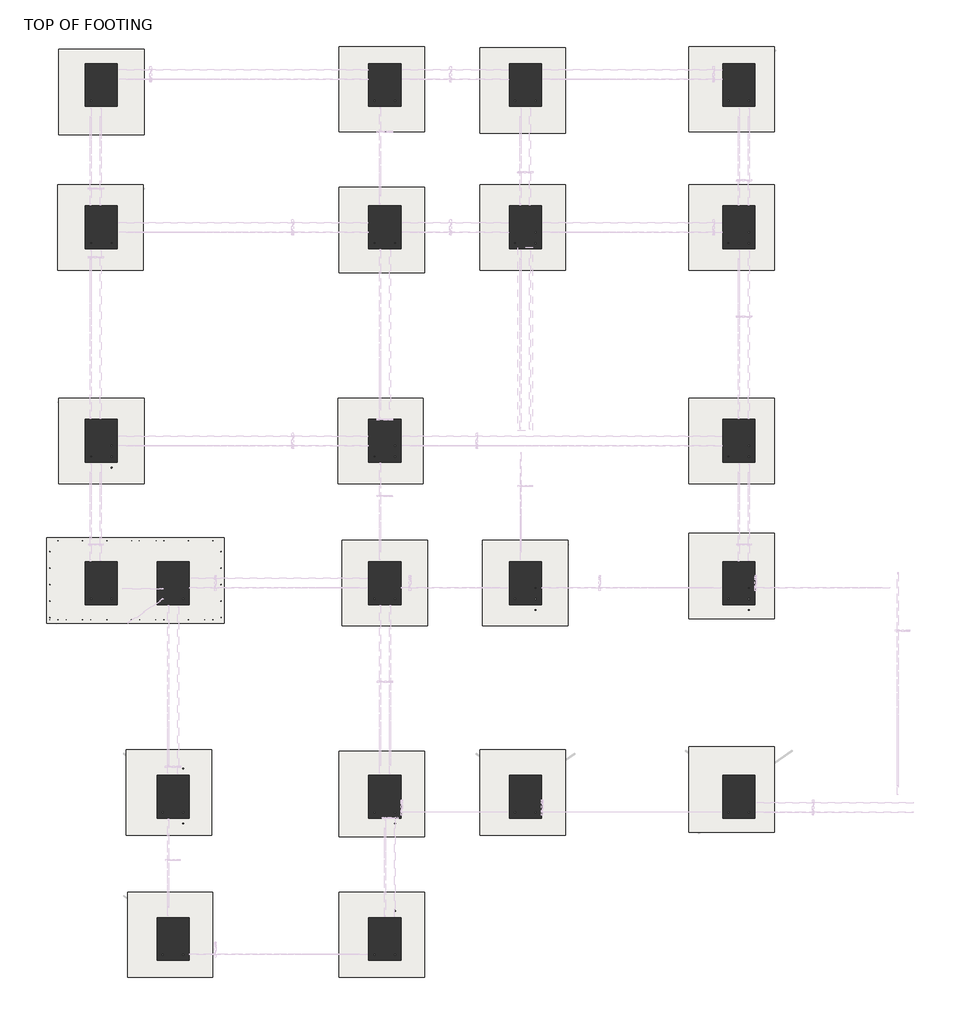
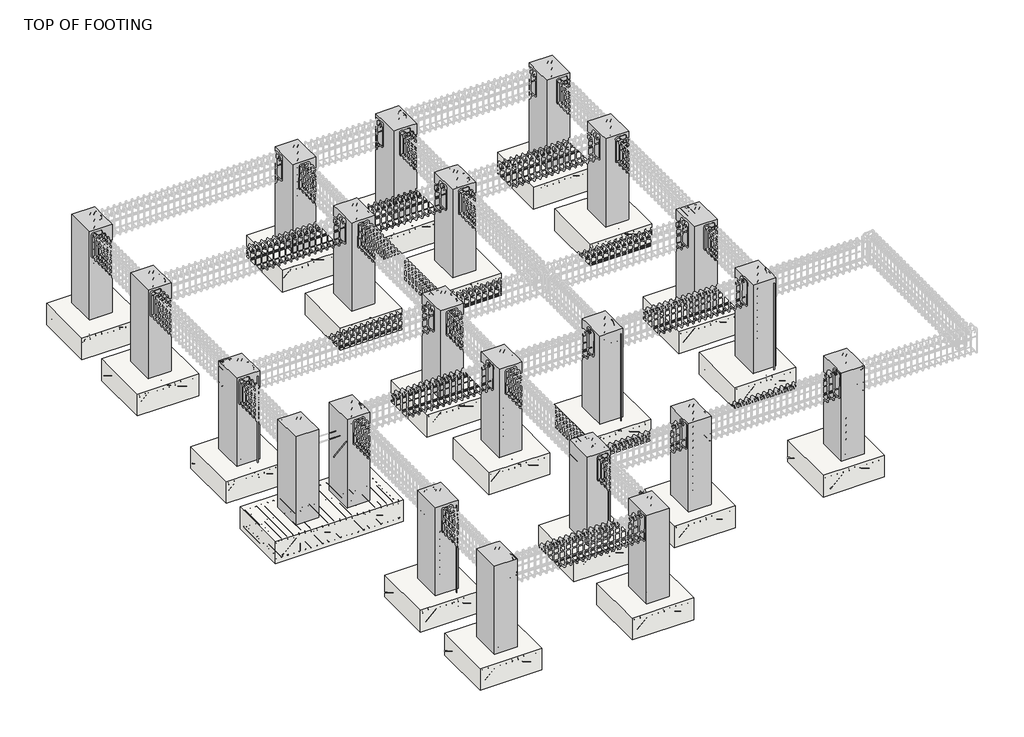
# One storey, part 1 of 17: 22 columns, 21 slabs.
"""IFC4 building model written with IfcOpenShell, lengths in millimetres."""

from ifc_helpers import new_model, si_unit, origin, place, context, project, spatial, faceted_brep, transform, mapped, element, save
from components import m_footing_rectangular_1200mmx1200mmx450mm_1789818b, m_footing_rectangular_1200mmx2500x450mm_3_75a58447

model = new_model("IFC4")

# Units and contexts
model_context = context("Model", 3, world=origin())
ifc_project = project(units=[si_unit("LENGTHUNIT", "METRE", prefix="MILLI")], contexts=[model_context])

# Site, building, storey
site = spatial("IfcSite", under=ifc_project)
building = spatial("IfcBuilding", under=site)
storey = spatial("IfcBuildingStorey", under=building, Name="TOP OF FOOTING", Elevation=-1828.8)

# Columns
placement = place(None, origin())
element("IfcColumn", 1, ObjectType="M_Concrete-Rectangular-Column : 450 x 600mm", at=placement, inside=storey, context=model_context, shape_type="Brep", body=[
    faceted_brep([(-4074.7920215, 9365.4757158, -1828.8), (-4074.7920215, 8765.4757158, -1828.8), (-4524.7920215, 8765.4757158, -1828.8), (-4524.7920215, 9365.4757158, -1828.8), (-4074.7920215, 9365.4757158, 0.0), (-4074.7920215, 9065.4757158, 0.0), (-4074.7920215, 8765.4757158, 0.0), (-4074.7920215, 8765.4757158, -300.0), (-4224.7920215, 8765.4757158, 0.0), (-4524.7920215, 8765.4757158, 0.0), (-4524.7920215, 9365.4757158, 0.0)], [[[0, 1, 2, 3]], [[1, 0, 4, 5, 6, 7]], [[2, 1, 7, 6, 8, 9]], [[3, 2, 9, 10]], [[0, 3, 10, 4]], [[10, 9, 8, 6, 5, 4]]]),
])
element("IfcColumn", 2, ObjectType="M_Concrete-Rectangular-Column : 450 x 600mm", at=placement, inside=storey, context=model_context, shape_type="Brep", body=[
    faceted_brep([(4887.1088658, 9365.4757158, -1828.8), (4887.1088658, 8765.4757158, -1828.8), (4437.1088658, 8765.4757158, -1828.8), (4437.1088658, 9365.4757158, -1828.8), (4887.1088658, 9365.4757158, 0.0), (4887.1088658, 8765.4757158, 0.0), (4587.1088658, 8765.4757158, 0.0), (4437.1088658, 8765.4757158, 0.0), (4437.1088658, 8765.4757158, -300.0), (4437.1088658, 9065.4757158, 0.0), (4437.1088658, 9365.4757158, 0.0)], [[[0, 1, 2, 3]], [[1, 0, 4, 5]], [[2, 1, 5, 6, 7, 8]], [[3, 2, 8, 7, 9, 10]], [[0, 3, 10, 4]], [[5, 4, 10, 9, 7, 6]]]),
])
element("IfcColumn", 3, ObjectType="M_Concrete-Rectangular-Column : 450 x 600mm", at=placement, inside=storey, context=model_context, shape_type="Brep", body=[
    faceted_brep([(1887.1088658, 9365.4757158, -1828.8), (1887.1088658, 8765.4757158, -1828.8), (1437.1088658, 8765.4757158, -1828.8), (1437.1088658, 9365.4757158, -1828.8), (1887.1088658, 9365.4757158, 0.0), (1887.1088658, 9065.4757158, 0.0), (1887.1088658, 8765.4757158, 0.0), (1887.1088658, 8765.4757158, -300.0), (1812.1088658, 8765.4757158, 0.0), (1512.1088658, 8765.4757158, 0.0), (1437.1088658, 8765.4757158, 0.0), (1437.1088658, 8765.4757158, -300.0), (1437.1088658, 9065.4757158, 0.0), (1437.1088658, 9365.4757158, 0.0)], [[[0, 1, 2, 3]], [[1, 0, 4, 5, 6, 7]], [[2, 1, 7, 6, 8, 9, 10, 11]], [[3, 2, 11, 10, 12, 13]], [[0, 3, 13, 4]], [[4, 13, 12, 10, 9, 8, 6, 5]]]),
])
element("IfcColumn", 4, ObjectType="M_Concrete-Rectangular-Column : 450 x 600mm", at=placement, inside=storey, context=model_context, shape_type="Brep", body=[
    faceted_brep([(-89.3669743, 9365.4757158, -1828.8), (-89.3669743, 8765.4757158, -1828.8), (-539.3669743, 8765.4757158, -1828.8), (-539.3669743, 9365.4757158, -1828.8), (-89.3669743, 9365.4757158, 0.0), (-89.3669743, 9065.4757158, 0.0), (-89.3669743, 8765.4757158, 0.0), (-89.3669743, 8765.4757158, -300.0), (-164.3669743, 8765.4757158, 0.0), (-464.3669743, 8765.4757158, 0.0), (-539.3669743, 8765.4757158, 0.0), (-539.3669743, 8765.4757158, -300.0), (-539.3669743, 9065.4757158, 0.0), (-539.3669743, 9365.4757158, 0.0)], [[[0, 1, 2, 3]], [[1, 0, 4, 5, 6, 7]], [[2, 1, 7, 6, 8, 9, 10, 11]], [[3, 2, 11, 10, 12, 13]], [[0, 3, 13, 4]], [[4, 13, 12, 10, 9, 8, 6, 5]]]),
])
element("IfcColumn", 5, ObjectType="M_Concrete-Rectangular-Column : 450 x 600mm", at=placement, inside=storey, context=model_context, shape_type="Brep", body=[
    faceted_brep([(-4074.7920215, 7365.4757158, -1828.8), (-4074.7920215, 6765.4757158, -1828.8), (-4524.7920215, 6765.4757158, -1828.8), (-4524.7920215, 7365.4757158, -1828.8), (-4074.7920215, 7365.4757158, -300.0), (-4074.7920215, 7365.4757158, 0.0), (-4074.7920215, 7215.4757158, 0.0), (-4074.7920215, 6915.4757158, 0.0), (-4074.7920215, 6765.4757158, 0.0), (-4074.7920215, 6765.4757158, -300.0), (-4224.7920215, 6765.4757158, 0.0), (-4524.7920215, 6765.4757158, 0.0), (-4524.7920215, 7365.4757158, 0.0), (-4224.7920215, 7365.4757158, 0.0)], [[[0, 1, 2, 3]], [[1, 0, 4, 5, 6, 7, 8, 9]], [[2, 1, 9, 8, 10, 11]], [[3, 2, 11, 12]], [[0, 3, 12, 13, 5, 4]], [[12, 11, 10, 8, 7, 6, 5, 13]]]),
])
element("IfcColumn", 6, ObjectType="M_Concrete-Rectangular-Column : 450 x 600mm", at=placement, inside=storey, context=model_context, shape_type="Brep", body=[
    faceted_brep([(-89.3669743, 7365.4757158, -1828.8), (-89.3669743, 6765.4757158, -1828.8), (-539.3669743, 6765.4757158, -1828.8), (-539.3669743, 7365.4757158, -1828.8), (-89.3669743, 7365.4757158, -300.0), (-89.3669743, 7365.4757158, 0.0), (-89.3669743, 7215.4757158, 0.0), (-89.3669743, 6915.4757158, 0.0), (-89.3669743, 6765.4757158, 0.0), (-89.3669743, 6765.4757158, -300.0), (-164.3669743, 6765.4757158, 0.0), (-464.3669743, 6765.4757158, 0.0), (-539.3669743, 6765.4757158, 0.0), (-539.3669743, 6765.4757158, -300.0), (-539.3669743, 6915.4757158, 0.0), (-539.3669743, 7215.4757158, 0.0), (-539.3669743, 7365.4757158, 0.0), (-539.3669743, 7365.4757158, -300.0), (-464.3669743, 7365.4757158, 0.0), (-164.3669743, 7365.4757158, 0.0)], [[[0, 1, 2, 3]], [[1, 0, 4, 5, 6, 7, 8, 9]], [[2, 1, 9, 8, 10, 11, 12, 13]], [[3, 2, 13, 12, 14, 15, 16, 17]], [[0, 3, 17, 16, 18, 19, 5, 4]], [[5, 19, 18, 16, 15, 14, 12, 11, 10, 8, 7, 6]]]),
])
element("IfcColumn", 7, ObjectType="M_Concrete-Rectangular-Column : 450 x 600mm", at=placement, inside=storey, context=model_context, shape_type="Brep", body=[
    faceted_brep([(1887.1088658, 7365.4757158, -1828.8), (1887.1088658, 6765.4757158, -1828.8), (1437.1088658, 6765.4757158, -1828.8), (1437.1088658, 7365.4757158, -1828.8), (1887.1088658, 7365.4757158, -300.0), (1887.1088658, 7365.4757158, 0.0), (1887.1088658, 7215.4757158, 0.0), (1887.1088658, 6915.4757158, 0.0), (1887.1088658, 6765.4757158, 0.0), (1887.1088658, 6765.4757158, -300.0), (1812.1088658, 6765.4757158, 0.0), (1512.1088658, 6765.4757158, 0.0), (1437.1088658, 6765.4757158, 0.0), (1437.1088658, 6765.4757158, -300.0), (1437.1088658, 6915.4757158, 0.0), (1437.1088658, 7215.4757158, 0.0), (1437.1088658, 7365.4757158, 0.0), (1437.1088658, 7365.4757158, -300.0), (1512.1088658, 7365.4757158, 0.0), (1812.1088658, 7365.4757158, 0.0)], [[[0, 1, 2, 3]], [[1, 0, 4, 5, 6, 7, 8, 9]], [[2, 1, 9, 8, 10, 11, 12, 13]], [[3, 2, 13, 12, 14, 15, 16, 17]], [[0, 3, 17, 16, 18, 19, 5, 4]], [[5, 19, 18, 16, 15, 14, 12, 11, 10, 8, 7, 6]]]),
])
element("IfcColumn", 8, ObjectType="M_Concrete-Rectangular-Column : 450 x 600mm", at=placement, inside=storey, context=model_context, shape_type="Brep", body=[
    faceted_brep([(4887.1088658, 7365.4757158, -1828.8), (4887.1088658, 6765.4757158, -1828.8), (4437.1088658, 6765.4757158, -1828.8), (4437.1088658, 7365.4757158, -1828.8), (4887.1088658, 7365.4757158, 0.0), (4887.1088658, 6765.4757158, 0.0), (4587.1088658, 6765.4757158, 0.0), (4437.1088658, 6765.4757158, 0.0), (4437.1088658, 6765.4757158, -300.0), (4437.1088658, 6915.4757158, 0.0), (4437.1088658, 7215.4757158, 0.0), (4437.1088658, 7365.4757158, 0.0), (4437.1088658, 7365.4757158, -300.0), (4587.1088658, 7365.4757158, 0.0)], [[[0, 1, 2, 3]], [[1, 0, 4, 5]], [[2, 1, 5, 6, 7, 8]], [[3, 2, 8, 7, 9, 10, 11, 12]], [[0, 3, 12, 11, 13, 4]], [[5, 4, 13, 11, 10, 9, 7, 6]]]),
])
element("IfcColumn", 9, ObjectType="M_Concrete-Rectangular-Column : 450 x 600mm", at=placement, inside=storey, context=model_context, shape_type="Brep", body=[
    faceted_brep([(-4074.7920215, 4365.4757158, -1828.8), (-4074.7920215, 3765.4757158, -1828.8), (-4524.7920215, 3765.4757158, -1828.8), (-4524.7920215, 4365.4757158, -1828.8), (-4074.7920215, 4365.4757158, -300.0), (-4074.7920215, 4365.4757158, 0.0), (-4074.7920215, 4215.4757158, 0.0), (-4074.7920215, 3915.4757158, 0.0), (-4074.7920215, 3765.4757158, 0.0), (-4074.7920215, 3765.4757158, -300.0), (-4224.7920215, 3765.4757158, 0.0), (-4524.7920215, 3765.4757158, 0.0), (-4524.7920215, 4365.4757158, 0.0), (-4224.7920215, 4365.4757158, 0.0)], [[[0, 1, 2, 3]], [[1, 0, 4, 5, 6, 7, 8, 9]], [[2, 1, 9, 8, 10, 11]], [[3, 2, 11, 12]], [[0, 3, 12, 13, 5, 4]], [[12, 11, 10, 8, 7, 6, 5, 13]]]),
])
element("IfcColumn", 10, ObjectType="M_Concrete-Rectangular-Column : 450 x 600mm", at=placement, inside=storey, context=model_context, shape_type="Brep", body=[
    faceted_brep([(4887.1088658, 4365.4757158, -1828.8), (4887.1088658, 3765.4757158, -1828.8), (4437.1088658, 3765.4757158, -1828.8), (4437.1088658, 4365.4757158, -1828.8), (4887.1088658, 4365.4757158, 0.0), (4887.1088658, 3765.4757158, 0.0), (4587.1088658, 3765.4757158, 0.0), (4437.1088658, 3765.4757158, 0.0), (4437.1088658, 3765.4757158, -300.0), (4437.1088658, 3915.4757158, 0.0), (4437.1088658, 4215.4757158, 0.0), (4437.1088658, 4365.4757158, 0.0), (4437.1088658, 4365.4757158, -300.0), (4587.1088658, 4365.4757158, 0.0)], [[[0, 1, 2, 3]], [[1, 0, 4, 5]], [[2, 1, 5, 6, 7, 8]], [[3, 2, 8, 7, 9, 10, 11, 12]], [[0, 3, 12, 11, 13, 4]], [[5, 4, 13, 11, 10, 9, 7, 6]]]),
])
element("IfcColumn", 11, ObjectType="M_Concrete-Rectangular-Column : 450 x 600mm", at=placement, inside=storey, context=model_context, shape_type="Brep", body=[
    faceted_brep([(-89.3669743, 4365.4757158, -1828.8), (-89.3669743, 3765.4757158, -1828.8), (-539.3669743, 3765.4757158, -1828.8), (-539.3669743, 4365.4757158, -1828.8), (-89.3669743, 4365.4757158, -300.0), (-89.3669743, 4365.4757158, 0.0), (-89.3669743, 4215.4757158, 0.0), (-89.3669743, 3915.4757158, 0.0), (-89.3669743, 3765.4757158, 0.0), (-89.3669743, 3765.4757158, -300.0), (-164.3669743, 3765.4757158, 0.0), (-464.3669743, 3765.4757158, 0.0), (-539.3669743, 3765.4757158, 0.0), (-539.3669743, 3765.4757158, -300.0), (-539.3669743, 3915.4757158, 0.0), (-539.3669743, 4215.4757158, 0.0), (-539.3669743, 4365.4757158, 0.0), (-539.3669743, 4365.4757158, -300.0), (-464.3669743, 4365.4757158, 0.0), (-164.3669743, 4365.4757158, 0.0)], [[[0, 1, 2, 3]], [[1, 0, 4, 5, 6, 7, 8, 9]], [[2, 1, 9, 8, 10, 11, 12, 13]], [[3, 2, 13, 12, 14, 15, 16, 17]], [[0, 3, 17, 16, 18, 19, 5, 4]], [[18, 16, 15, 14, 12, 11, 10, 8, 7, 6, 5, 19]]]),
])
element("IfcColumn", 12, ObjectType="M_Concrete-Rectangular-Column : 450 x 600mm", at=placement, inside=storey, context=model_context, shape_type="Brep", body=[
    faceted_brep([(-4074.7920215, 2365.4757158, -1828.8), (-4074.7920215, 1765.4757158, -1828.8), (-4524.7920215, 1765.4757158, -1828.8), (-4524.7920215, 2365.4757158, -1828.8), (-4074.7920215, 2365.4757158, -300.0), (-4074.7920215, 2365.4757158, 0.0), (-4074.7920215, 2215.4757158, 0.0), (-4074.7920215, 1765.4757158, 0.0), (-4524.7920215, 1765.4757158, 0.0), (-4524.7920215, 2365.4757158, 0.0), (-4224.7920215, 2365.4757158, 0.0)], [[[0, 1, 2, 3]], [[1, 0, 4, 5, 6, 7]], [[2, 1, 7, 8]], [[3, 2, 8, 9]], [[0, 3, 9, 10, 5, 4]], [[8, 7, 6, 5, 10, 9]]]),
])
element("IfcColumn", 13, ObjectType="M_Concrete-Rectangular-Column : 450 x 600mm", at=placement, inside=storey, context=model_context, shape_type="Brep", body=[
    faceted_brep([(-3067.007124, 2365.4757158, -1828.8), (-3067.007124, 1765.4757158, -1828.8), (-3517.007124, 1765.4757158, -1828.8), (-3517.007124, 2365.4757158, -1828.8), (-3067.007124, 2365.4757158, -300.0), (-3067.007124, 2365.4757158, 0.0), (-3067.007124, 2215.4757158, 0.0), (-3067.007124, 1915.4757158, 0.0), (-3067.007124, 1765.4757158, 0.0), (-3067.007124, 1765.4757158, -300.0), (-3142.007124, 1765.4757158, 0.0), (-3517.007124, 1765.4757158, 0.0), (-3517.007124, 2215.4757158, 0.0), (-3517.007124, 2365.4757158, 0.0), (-3517.007124, 2365.4757158, -300.0)], [[[0, 1, 2, 3]], [[1, 0, 4, 5, 6, 7, 8, 9]], [[2, 1, 9, 8, 10, 11]], [[3, 2, 11, 12, 13, 14]], [[0, 3, 14, 13, 5, 4]], [[5, 13, 12, 11, 10, 8, 7, 6]]]),
])
element("IfcColumn", 14, ObjectType="M_Concrete-Rectangular-Column : 450 x 600mm", at=placement, inside=storey, context=model_context, shape_type="Brep", body=[
    faceted_brep([(-89.3669743, 2365.4757158, -1828.8), (-89.3669743, 1765.4757158, -1828.8), (-539.3669743, 1765.4757158, -1828.8), (-539.3669743, 2365.4757158, -1828.8), (-89.3669743, 2365.4757158, -300.0), (-89.3669743, 2365.4757158, 0.0), (-89.3669743, 2215.4757158, 0.0), (-89.3669743, 1915.4757158, 0.0), (-89.3669743, 1765.4757158, 0.0), (-89.3669743, 1765.4757158, -300.0), (-164.3669743, 1765.4757158, 0.0), (-464.3669743, 1765.4757158, 0.0), (-539.3669743, 1765.4757158, 0.0), (-539.3669743, 1765.4757158, -300.0), (-539.3669743, 1915.4757158, 0.0), (-539.3669743, 2215.4757158, 0.0), (-539.3669743, 2365.4757158, 0.0), (-539.3669743, 2365.4757158, -300.0), (-464.3669743, 2365.4757158, 0.0), (-164.3669743, 2365.4757158, 0.0)], [[[0, 1, 2, 3]], [[1, 0, 4, 5, 6, 7, 8, 9]], [[2, 1, 9, 8, 10, 11, 12, 13]], [[3, 2, 13, 12, 14, 15, 16, 17]], [[0, 3, 17, 16, 18, 19, 5, 4]], [[18, 16, 15, 14, 12, 11, 10, 8, 7, 6, 5, 19]]]),
])
element("IfcColumn", 15, ObjectType="M_Concrete-Rectangular-Column : 450 x 600mm", at=placement, inside=storey, context=model_context, shape_type="Brep", body=[
    faceted_brep([(4887.1088658, 2365.4757158, -1828.8), (4887.1088658, 1765.4757158, -1828.8), (4437.1088658, 1765.4757158, -1828.8), (4437.1088658, 2365.4757158, -1828.8), (4887.1088658, 2365.4757158, 0.0), (4887.1088658, 1915.4757158, 0.0), (4887.1088658, 1765.4757158, 0.0), (4887.1088658, 1765.4757158, -300.0), (4437.1088658, 1765.4757158, 0.0), (4437.1088658, 1765.4757158, -300.0), (4437.1088658, 1915.4757158, 0.0), (4437.1088658, 2215.4757158, 0.0), (4437.1088658, 2365.4757158, 0.0), (4437.1088658, 2365.4757158, -300.0), (4587.1088658, 2365.4757158, 0.0)], [[[0, 1, 2, 3]], [[1, 0, 4, 5, 6, 7]], [[2, 1, 7, 6, 8, 9]], [[3, 2, 9, 8, 10, 11, 12, 13]], [[0, 3, 13, 12, 14, 4]], [[8, 6, 5, 4, 14, 12, 11, 10]]]),
])
element("IfcColumn", 16, ObjectType="M_Concrete-Rectangular-Column : 450 x 600mm", at=placement, inside=storey, context=model_context, shape_type="Brep", body=[
    faceted_brep([(1887.1088658, 2365.4757158, -1828.8), (1887.1088658, 1765.4757158, -1828.8), (1437.1088658, 1765.4757158, -1828.8), (1437.1088658, 2365.4757158, -1828.8), (1887.1088658, 2365.4757158, -300.0), (1887.1088658, 2365.4757158, 0.0), (1887.1088658, 2215.4757158, 0.0), (1887.1088658, 1915.4757158, 0.0), (1887.1088658, 1765.4757158, 0.0), (1887.1088658, 1765.4757158, -300.0), (1437.1088658, 1765.4757158, 0.0), (1437.1088658, 1765.4757158, -300.0), (1437.1088658, 1915.4757158, 0.0), (1437.1088658, 2215.4757158, 0.0), (1437.1088658, 2365.4757158, 0.0), (1437.1088658, 2365.4757158, -300.0), (1512.1088658, 2365.4757158, 0.0), (1812.1088658, 2365.4757158, 0.0)], [[[0, 1, 2, 3]], [[1, 0, 4, 5, 6, 7, 8, 9]], [[2, 1, 9, 8, 10, 11]], [[3, 2, 11, 10, 12, 13, 14, 15]], [[0, 3, 15, 14, 16, 17, 5, 4]], [[10, 8, 7, 6, 5, 17, 16, 14, 13, 12]]]),
])
element("IfcColumn", 17, ObjectType="M_Concrete-Rectangular-Column : 450 x 600mm", at=placement, inside=storey, context=model_context, shape_type="Brep", body=[
    faceted_brep([(-3067.007124, -634.5242842, -1828.8), (-3067.007124, -1234.5242842, -1828.8), (-3517.007124, -1234.5242842, -1828.8), (-3517.007124, -634.5242842, -1828.8), (-3067.007124, -634.5242842, -300.0), (-3067.007124, -634.5242842, 0.0), (-3067.007124, -1234.5242842, 0.0), (-3067.007124, -1234.5242842, -300.0), (-3142.007124, -1234.5242842, 0.0), (-3517.007124, -1234.5242842, 0.0), (-3517.007124, -634.5242842, 0.0), (-3142.007124, -634.5242842, 0.0)], [[[0, 1, 2, 3]], [[1, 0, 4, 5, 6, 7]], [[2, 1, 7, 6, 8, 9]], [[3, 2, 9, 10]], [[0, 3, 10, 11, 5, 4]], [[6, 5, 11, 10, 9, 8]]]),
])
element("IfcColumn", 18, ObjectType="M_Concrete-Rectangular-Column : 450 x 600mm", at=placement, inside=storey, context=model_context, shape_type="Brep", body=[
    faceted_brep([(4887.1088658, -634.5242842, -1828.8), (4887.1088658, -1234.5242842, -1828.8), (4437.1088658, -1234.5242842, -1828.8), (4437.1088658, -634.5242842, -1828.8), (4887.1088658, -634.5242842, -300.0), (4887.1088658, -634.5242842, 0.0), (4887.1088658, -934.5242842, 0.0), (4887.1088658, -1234.5242842, 0.0), (4437.1088658, -1234.5242842, 0.0), (4437.1088658, -934.5242842, 0.0), (4437.1088658, -634.5242842, 0.0), (4437.1088658, -634.5242842, -300.0)], [[[0, 1, 2, 3]], [[1, 0, 4, 5, 6, 7]], [[2, 1, 7, 8]], [[3, 2, 8, 9, 10, 11]], [[0, 3, 11, 10, 5, 4]], [[8, 7, 6, 5, 10, 9]]]),
])
element("IfcColumn", 19, ObjectType="M_Concrete-Rectangular-Column : 450 x 600mm", at=placement, inside=storey, context=model_context, shape_type="Brep", body=[
    faceted_brep([(1887.1088658, -634.5242842, -1828.8), (1887.1088658, -1234.5242842, -1828.8), (1437.1088658, -1234.5242842, -1828.8), (1437.1088658, -634.5242842, -1828.8), (1887.1088658, -634.5242842, -300.0), (1887.1088658, -634.5242842, 0.0), (1887.1088658, -934.5242842, 0.0), (1887.1088658, -1234.5242842, 0.0), (1437.1088658, -1234.5242842, 0.0), (1437.1088658, -934.5242842, 0.0), (1437.1088658, -634.5242842, 0.0), (1437.1088658, -634.5242842, -300.0)], [[[0, 1, 2, 3]], [[1, 0, 4, 5, 6, 7]], [[2, 1, 7, 8]], [[3, 2, 8, 9, 10, 11]], [[0, 3, 11, 10, 5, 4]], [[8, 7, 6, 5, 10, 9]]]),
])
element("IfcColumn", 20, ObjectType="M_Concrete-Rectangular-Column : 450 x 600mm", at=placement, inside=storey, context=model_context, shape_type="Brep", body=[
    faceted_brep([(-89.3669743, -634.5242842, -1828.8), (-89.3669743, -1234.5242842, -1828.8), (-539.3669743, -1234.5242842, -1828.8), (-539.3669743, -634.5242842, -1828.8), (-89.3669743, -634.5242842, -300.0), (-89.3669743, -634.5242842, 0.0), (-89.3669743, -934.5242842, 0.0), (-89.3669743, -1234.5242842, 0.0), (-389.3669743, -1234.5242842, 0.0), (-539.3669743, -1234.5242842, 0.0), (-539.3669743, -1234.5242842, -300.0), (-539.3669743, -634.5242842, 0.0), (-539.3669743, -634.5242842, -300.0), (-464.3669743, -634.5242842, 0.0), (-164.3669743, -634.5242842, 0.0)], [[[0, 1, 2, 3]], [[1, 0, 4, 5, 6, 7]], [[2, 1, 7, 8, 9, 10]], [[3, 2, 10, 9, 11, 12]], [[0, 3, 12, 11, 13, 14, 5, 4]], [[11, 9, 8, 7, 6, 5, 14, 13]]]),
])
element("IfcColumn", 21, ObjectType="M_Concrete-Rectangular-Column : 450 x 600mm", at=placement, inside=storey, context=model_context, shape_type="Brep", body=[
    faceted_brep([(-3067.007124, -2634.5242842, -1828.8), (-3067.007124, -3234.5242842, -1828.8), (-3517.007124, -3234.5242842, -1828.8), (-3517.007124, -2634.5242842, -1828.8), (-3067.007124, -2634.5242842, -300.0), (-3067.007124, -2634.5242842, 0.0), (-3067.007124, -2934.5242842, 0.0), (-3067.007124, -3234.5242842, 0.0), (-3517.007124, -3234.5242842, 0.0), (-3517.007124, -2634.5242842, 0.0), (-3142.007124, -2634.5242842, 0.0)], [[[0, 1, 2, 3]], [[1, 0, 4, 5, 6, 7]], [[2, 1, 7, 8]], [[3, 2, 8, 9]], [[0, 3, 9, 10, 5, 4]], [[8, 7, 6, 5, 10, 9]]]),
])
element("IfcColumn", 22, ObjectType="M_Concrete-Rectangular-Column : 450 x 600mm", at=placement, inside=storey, context=model_context, shape_type="Brep", body=[
    faceted_brep([(-89.3669743, -2634.5242842, -1828.8), (-89.3669743, -3234.5242842, -1828.8), (-539.3669743, -3234.5242842, -1828.8), (-539.3669743, -2634.5242842, -1828.8), (-89.3669743, -2634.5242842, 0.0), (-89.3669743, -3234.5242842, 0.0), (-539.3669743, -3234.5242842, 0.0), (-539.3669743, -2934.5242842, 0.0), (-539.3669743, -2634.5242842, 0.0), (-539.3669743, -2634.5242842, -300.0), (-389.3669743, -2634.5242842, 0.0)], [[[0, 1, 2, 3]], [[1, 0, 4, 5]], [[2, 1, 5, 6]], [[3, 2, 6, 7, 8, 9]], [[0, 3, 9, 8, 10, 4]], [[5, 4, 10, 8, 7, 6]]]),
])

# Slabs
m_footing_rectangular_1200mmx1200mmx450mm_shape = m_footing_rectangular_1200mmx1200mmx450mm_1789818b(model_context)
element("IfcSlab", 23, ObjectType="M_Footing-Rectangular : 1200MMX1200MMX450MM", at=placement, inside=storey, context=model_context, shape_type="MappedRepresentation", body=[
    mapped(m_footing_rectangular_1200mmx1200mmx450mm_shape, transform((-4299.7920215, 8965.4757158, -1828.8), x_axis=(1.0, 0.0, 0.0), y_axis=(0.0, 1.0, 0.0), z_axis=(0.0, 0.0, 1.0))),
])
element("IfcSlab", 24, ObjectType="M_Footing-Rectangular : 1200MMX1200MMX450MM", at=placement, inside=storey, context=model_context, shape_type="MappedRepresentation", body=[
    mapped(m_footing_rectangular_1200mmx1200mmx450mm_shape, transform((-354.3669743, 9005.4757158, -1828.8), x_axis=(1.0, 0.0, 0.0), y_axis=(0.0, 1.0, 0.0), z_axis=(0.0, 0.0, 1.0))),
])
element("IfcSlab", 25, ObjectType="M_Footing-Rectangular : 1200MMX1200MMX450MM", at=placement, inside=storey, context=model_context, shape_type="MappedRepresentation", body=[
    mapped(m_footing_rectangular_1200mmx1200mmx450mm_shape, transform((1622.1088658, 8985.4757158, -1828.8), x_axis=(1.0, 0.0, 0.0), y_axis=(0.0, 1.0, 0.0), z_axis=(0.0, 0.0, 1.0))),
])
element("IfcSlab", 26, ObjectType="M_Footing-Rectangular : 1200MMX1200MMX450MM", at=placement, inside=storey, context=model_context, shape_type="MappedRepresentation", body=[
    mapped(m_footing_rectangular_1200mmx1200mmx450mm_shape, transform((4562.1088658, 9005.4757158, -1828.8), x_axis=(1.0, 0.0, 0.0), y_axis=(0.0, 1.0, 0.0), z_axis=(0.0, 0.0, 1.0))),
])
element("IfcSlab", 27, ObjectType="M_Footing-Rectangular : 1200MMX1200MMX450MM", at=placement, inside=storey, context=model_context, shape_type="MappedRepresentation", body=[
    mapped(m_footing_rectangular_1200mmx1200mmx450mm_shape, transform((-4312.007124, 7065.4757158, -1828.8), x_axis=(1.0, 0.0, 0.0), y_axis=(0.0, 1.0, 0.0), z_axis=(0.0, 0.0, 1.0))),
])
element("IfcSlab", 28, ObjectType="M_Footing-Rectangular : 1200MMX1200MMX450MM", at=placement, inside=storey, context=model_context, shape_type="MappedRepresentation", body=[
    mapped(m_footing_rectangular_1200mmx1200mmx450mm_shape, transform((-4299.7920215, 4065.4757158, -1828.8), x_axis=(1.0, 0.0, 0.0), y_axis=(0.0, 1.0, 0.0), z_axis=(0.0, 0.0, 1.0))),
])
element("IfcSlab", 29, ObjectType="M_Footing-Rectangular : 1200MMX1200MMX450MM", at=placement, inside=storey, context=model_context, shape_type="MappedRepresentation", body=[
    mapped(m_footing_rectangular_1200mmx1200mmx450mm_shape, transform((-314.3669743, 2065.4757158, -1828.8), x_axis=(1.0, 0.0, 0.0), y_axis=(0.0, 1.0, 0.0), z_axis=(0.0, 0.0, 1.0))),
])
element("IfcSlab", 30, ObjectType="M_Footing-Rectangular : 1200MMX1200MMX450MM", at=placement, inside=storey, context=model_context, shape_type="MappedRepresentation", body=[
    mapped(m_footing_rectangular_1200mmx1200mmx450mm_shape, transform((1662.1088658, 2065.4757158, -1828.8), x_axis=(1.0, 0.0, 0.0), y_axis=(0.0, 1.0, 0.0), z_axis=(0.0, 0.0, 1.0))),
])
element("IfcSlab", 31, ObjectType="M_Footing-Rectangular : 1200MMX1200MMX450MM", at=placement, inside=storey, context=model_context, shape_type="MappedRepresentation", body=[
    mapped(m_footing_rectangular_1200mmx1200mmx450mm_shape, transform((4562.1088658, 2165.4757158, -1828.8), x_axis=(1.0, 0.0, 0.0), y_axis=(0.0, 1.0, 0.0), z_axis=(0.0, 0.0, 1.0))),
])
element("IfcSlab", 32, ObjectType="M_Footing-Rectangular : 1200MMX1200MMX450MM", at=placement, inside=storey, context=model_context, shape_type="MappedRepresentation", body=[
    mapped(m_footing_rectangular_1200mmx1200mmx450mm_shape, transform((4562.1088658, -834.5242842, -1828.8), x_axis=(1.0, 0.0, 0.0), y_axis=(0.0, 1.0, 0.0), z_axis=(0.0, 0.0, 1.0))),
])
element("IfcSlab", 33, ObjectType="M_Footing-Rectangular : 1200MMX1200MMX450MM", at=placement, inside=storey, context=model_context, shape_type="MappedRepresentation", body=[
    mapped(m_footing_rectangular_1200mmx1200mmx450mm_shape, transform((1622.1088658, -874.5242842, -1828.8), x_axis=(1.0, 0.0, 0.0), y_axis=(0.0, 1.0, 0.0), z_axis=(0.0, 0.0, 1.0))),
])
element("IfcSlab", 34, ObjectType="M_Footing-Rectangular : 1200MMX1200MMX450MM", at=placement, inside=storey, context=model_context, shape_type="MappedRepresentation", body=[
    mapped(m_footing_rectangular_1200mmx1200mmx450mm_shape, transform((-354.3669743, -894.5242842, -1828.8), x_axis=(1.0, 0.0, 0.0), y_axis=(0.0, 1.0, 0.0), z_axis=(0.0, 0.0, 1.0))),
])
element("IfcSlab", 35, ObjectType="M_Footing-Rectangular : 1200MMX1200MMX450MM", at=placement, inside=storey, context=model_context, shape_type="MappedRepresentation", body=[
    mapped(m_footing_rectangular_1200mmx1200mmx450mm_shape, transform((-3352.007124, -874.5242842, -1828.8), x_axis=(1.0, 0.0, 0.0), y_axis=(0.0, 1.0, 0.0), z_axis=(0.0, 0.0, 1.0))),
])
element("IfcSlab", 36, ObjectType="M_Footing-Rectangular : 1200MMX1200MMX450MM", at=placement, inside=storey, context=model_context, shape_type="MappedRepresentation", body=[
    mapped(m_footing_rectangular_1200mmx1200mmx450mm_shape, transform((-3332.007124, -2874.5242842, -1828.8), x_axis=(1.0, 0.0, 0.0), y_axis=(0.0, 1.0, 0.0), z_axis=(0.0, 0.0, 1.0))),
])
element("IfcSlab", 37, ObjectType="M_Footing-Rectangular : 1200MMX1200MMX450MM", at=placement, inside=storey, context=model_context, shape_type="MappedRepresentation", body=[
    mapped(m_footing_rectangular_1200mmx1200mmx450mm_shape, transform((-354.3669743, -2874.5242842, -1828.8), x_axis=(1.0, 0.0, 0.0), y_axis=(0.0, 1.0, 0.0), z_axis=(0.0, 0.0, 1.0))),
])
element("IfcSlab", 38, ObjectType="M_Footing-Rectangular : 1200MMX1200MMX450MM", at=placement, inside=storey, context=model_context, shape_type="MappedRepresentation", body=[
    mapped(m_footing_rectangular_1200mmx1200mmx450mm_shape, transform((-374.3669743, 4065.4757158, -1828.8), x_axis=(1.0, 0.0, 0.0), y_axis=(0.0, 1.0, 0.0), z_axis=(0.0, 0.0, 1.0))),
])
element("IfcSlab", 39, ObjectType="M_Footing-Rectangular : 1200MMX1200MMX450MM", at=placement, inside=storey, context=model_context, shape_type="MappedRepresentation", body=[
    mapped(m_footing_rectangular_1200mmx1200mmx450mm_shape, transform((4562.1088658, 4065.4757158, -1828.8), x_axis=(1.0, 0.0, 0.0), y_axis=(0.0, 1.0, 0.0), z_axis=(0.0, 0.0, 1.0))),
])
element("IfcSlab", 40, ObjectType="M_Footing-Rectangular : 1200MMX1200MMX450MM", at=placement, inside=storey, context=model_context, shape_type="MappedRepresentation", body=[
    mapped(m_footing_rectangular_1200mmx1200mmx450mm_shape, transform((4562.1088658, 7065.4757158, -1828.8), x_axis=(1.0, 0.0, 0.0), y_axis=(0.0, 1.0, 0.0), z_axis=(0.0, 0.0, 1.0))),
])
element("IfcSlab", 41, ObjectType="M_Footing-Rectangular : 1200MMX1200MMX450MM", at=placement, inside=storey, context=model_context, shape_type="MappedRepresentation", body=[
    mapped(m_footing_rectangular_1200mmx1200mmx450mm_shape, transform((1622.1088658, 7065.4757158, -1828.8), x_axis=(1.0, 0.0, 0.0), y_axis=(0.0, 1.0, 0.0), z_axis=(0.0, 0.0, 1.0))),
])
element("IfcSlab", 42, ObjectType="M_Footing-Rectangular : 1200MMX1200MMX450MM", at=placement, inside=storey, context=model_context, shape_type="MappedRepresentation", body=[
    mapped(m_footing_rectangular_1200mmx1200mmx450mm_shape, transform((-354.3669743, 7025.4757158, -1828.8), x_axis=(1.0, 0.0, 0.0), y_axis=(0.0, 1.0, 0.0), z_axis=(0.0, 0.0, 1.0))),
])
m_footing_rectangular_1200mmx2500x450mm_3_shape = m_footing_rectangular_1200mmx2500x450mm_3_75a58447(model_context)
element("IfcSlab", 43, ObjectType="M_Footing-Rectangular : 1200MMX2500X450MM 3", at=placement, inside=storey, context=model_context, shape_type="MappedRepresentation", body=[
    mapped(m_footing_rectangular_1200mmx2500x450mm_3_shape, transform((-3819.7920215, 2105.4757158, -1828.8), x_axis=(0.0, 1.0, 0.0), y_axis=(-1.0, 0.0, 0.0), z_axis=(0.0, 0.0, 1.0))),
])

save(model, "model.ifc")

# Revit data of these elements
# Grids (mm)
#   "1": line (-4299.792, -7551.18) -> (-4299.792, 10278.991)
#   "3": line (-1299.792, -7551.18) -> (-1299.792, 10278.991)
#   "4": line (-314.367, -7551.18) -> (-314.367, 10429.888)
#   "5": line (1662.109, -7551.18) -> (1662.109, 11644.031)
#   "6": line (4662.109, -7551.18) -> (4662.109, 11644.031)
#   "2": line (-3292.007, -7551.18) -> (-3292.007, 11644.031)
#   "A": line (9910.38, 9065.476) -> (-6361.637, 9065.476)
#   "B": line (9910.38, 7065.476) -> (-6361.637, 7065.476)
#   "C": line (9910.38, 4065.476) -> (-6361.637, 4065.476)
#   "D": line (9910.38, 2065.476) -> (-6361.637, 2065.476)
#   "E": line (9910.38, -934.524) -> (-6361.637, -934.524)
#   "F": line (9910.38, -2934.524) -> (-6361.637, -2934.524)
# Type "M_Concrete-Rectangular-Column : 450 x 600mm"
#   b = 450 mm
#   h = 600 mm
#   Structural Material [instance default] = Concrete, Cast-in-Place gray
# Type "M_Footing-Rectangular : 1200MMX1200MMX450MM"
#   Width = 1200 mm
#   Length = 1200 mm
#   Foundation Thickness = 450 mm
#   Structural Material [instance default] = Concrete, Cast-in-Place gray
#   Assembly Code = ""
# Type "M_Footing-Rectangular : 1200MMX2500X450MM 3"
#   Width = 1200 mm
#   Length = 2500 mm
#   Foundation Thickness = 450 mm
#   Structural Material [instance default] = Concrete, Cast-in-Place gray
#   Assembly Code = ""
# Elements 1, 2, 3, 4, 5, 6, 7, 8, 9, 10, 11, 12, 13, 14, 15, 16, 17, 18, 19, 20, 21, 22 (IfcColumn, "M_Concrete-Rectangular-Column : 450 x 600mm")
#   Structural Material = Concrete, Cast-in-Place gray
#   Phase Created = New Construction
#   Materials on its faces: "Concrete, Cast-in-Place gray"
# Elements 23, 24, 25, 26, 27, 28, 29, 30, 31, 32, 33, 34, 35, 36, 37, 38, 39, 40, 41, 42 (IfcSlab, "M_Footing-Rectangular : 1200MMX1200MMX450MM")
#   Structural Material = Concrete, Cast-in-Place gray
#   Phase Created = New Construction
#   Materials on its faces: "Concrete, Cast-in-Place gray"
# Element 43 (IfcSlab, "M_Footing-Rectangular : 1200MMX2500X450MM 3")
#   Structural Material = Concrete, Cast-in-Place gray
#   Phase Created = New Construction
#   Materials on its faces: "Concrete, Cast-in-Place gray"
# Materials
#   "Concrete, Cast-in-Place gray": class "Concrete", colour RGB 192 192 192, transparency 0, Description = "Cast-in-place concrete", Cost = 0
